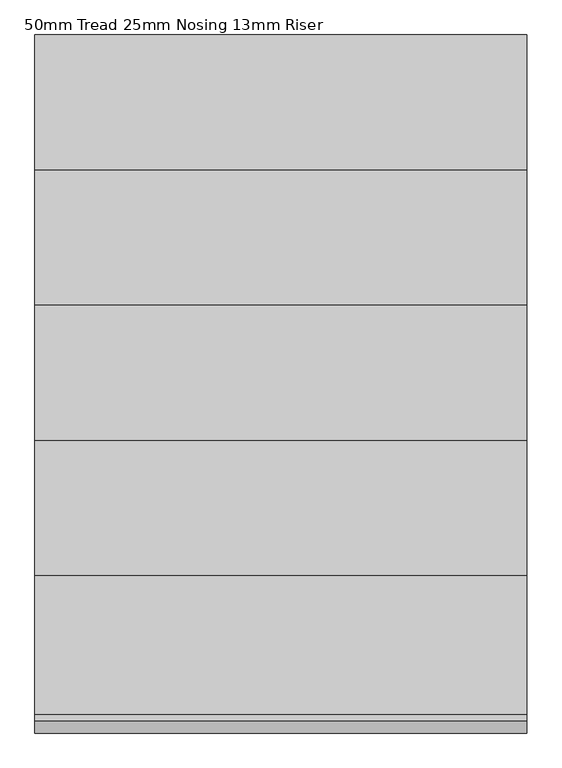
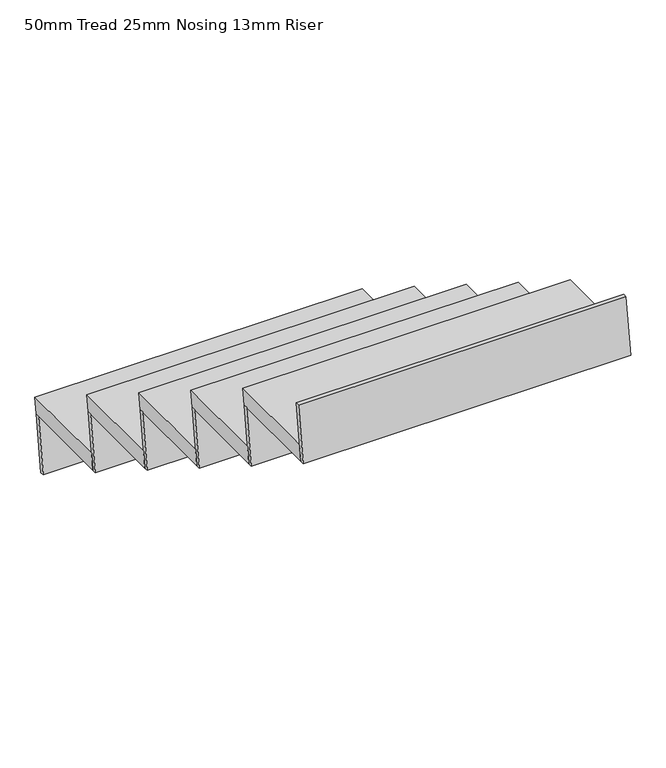
"""IFC4 building model written with IfcOpenShell, lengths in millimetres: stair flight geometry, 50mm Tread 25mm Nosing 13mm Riser."""

from ifc_helpers import new_model, si_unit, frame, origin, place, context, project, spatial, polyline, outline, extrude, source, transform, mapped, element, save


def stair_flight_50mm_tread_25mm_nosing_13mm_riser_46b24cc8(model_context):
    return source(origin(), model_context, "Body", "SweptSolid", [
        extrude(outline(polyline([(2452.4280728, 1739.1304348), (2752.4280728, 1739.1304348), (2745.2405728, 1689.1304348), (2445.2405728, 1689.1304348), (2452.4280728, 1739.1304348)])), frame((-10585.5805681, 0.0, 0.0), z_axis=(1.0, 0.0, 0.0), x_axis=(0.0, 1.0, 0.0)), (0.0, 0.0, 1.0), 1000.0257813),
        extrude(outline(polyline([(2745.2405728, 1689.1304348), (2720.2405728, 1515.2173913), (2707.6120828, 1515.2173913), (2732.6120828, 1689.1304348), (2745.2405728, 1689.1304348)])), frame((-10585.5805681, 0.0, 0.0), z_axis=(1.0, 0.0, 0.0), x_axis=(0.0, 1.0, 0.0)), (0.0, 0.0, 1.0), 1000.0257813),
        extrude(outline(polyline([(2470.2405728, 1863.0434783), (2445.2405728, 1689.1304348), (2432.6120828, 1689.1304348), (2457.6120828, 1863.0434783), (2470.2405728, 1863.0434783)])), frame((-10585.5805681, 0.0, 0.0), z_axis=(1.0, 0.0, 0.0), x_axis=(0.0, 1.0, 0.0)), (0.0, 0.0, 1.0), 1000.0257813),
        extrude(outline(polyline([(2177.4280728, 1913.0434783), (2477.4280728, 1913.0434783), (2470.2405728, 1863.0434783), (2170.2405728, 1863.0434783), (2177.4280728, 1913.0434783)])), frame((-10585.5805681, 0.0, 0.0), z_axis=(1.0, 0.0, 0.0), x_axis=(0.0, 1.0, 0.0)), (0.0, 0.0, 1.0), 1000.0257813),
        extrude(outline(polyline([(2195.2405728, 2036.9565217), (2170.2405728, 1863.0434783), (2157.6120828, 1863.0434783), (2182.6120828, 2036.9565217), (2195.2405728, 2036.9565217)])), frame((-10585.5805681, 0.0, 0.0), z_axis=(1.0, 0.0, 0.0), x_axis=(0.0, 1.0, 0.0)), (0.0, 0.0, 1.0), 1000.0257813),
        extrude(outline(polyline([(1902.4280728, 2086.9565217), (2202.4280728, 2086.9565217), (2195.2405728, 2036.9565217), (1895.2405728, 2036.9565217), (1902.4280728, 2086.9565217)])), frame((-10585.5805681, 0.0, 0.0), z_axis=(1.0, 0.0, 0.0), x_axis=(0.0, 1.0, 0.0)), (0.0, 0.0, 1.0), 1000.0257813),
        extrude(outline(polyline([(1920.2405728, 2210.8695652), (1895.2405728, 2036.9565217), (1882.6120828, 2036.9565217), (1907.6120828, 2210.8695652), (1920.2405728, 2210.8695652)])), frame((-10585.5805681, 0.0, 0.0), z_axis=(1.0, 0.0, 0.0), x_axis=(0.0, 1.0, 0.0)), (0.0, 0.0, 1.0), 1000.0257813),
        extrude(outline(polyline([(1627.4280728, 2260.8695652), (1927.4280728, 2260.8695652), (1920.2405728, 2210.8695652), (1620.2405728, 2210.8695652), (1627.4280728, 2260.8695652)])), frame((-10585.5805681, 0.0, 0.0), z_axis=(1.0, 0.0, 0.0), x_axis=(0.0, 1.0, 0.0)), (0.0, 0.0, 1.0), 1000.0257813),
        extrude(outline(polyline([(1645.2405728, 2384.7826087), (1620.2405728, 2210.8695652), (1607.6120828, 2210.8695652), (1632.6120828, 2384.7826087), (1645.2405728, 2384.7826087)])), frame((-10585.5805681, 0.0, 0.0), z_axis=(1.0, 0.0, 0.0), x_axis=(0.0, 1.0, 0.0)), (0.0, 0.0, 1.0), 1000.0257813),
        extrude(outline(polyline([(1370.2405728, 2558.6956522), (1345.2405728, 2384.7826087), (1332.6120828, 2384.7826087), (1357.6120828, 2558.6956522), (1370.2405728, 2558.6956522)])), frame((-10585.5805681, 0.0, 0.0), z_axis=(1.0, 0.0, 0.0), x_axis=(0.0, 1.0, 0.0)), (0.0, 0.0, 1.0), 1000.0257813),
        extrude(outline(polyline([(1352.4280728, 2434.7826087), (1652.4280728, 2434.7826087), (1645.2405728, 2384.7826087), (1345.2405728, 2384.7826087), (1352.4280728, 2434.7826087)])), frame((-10585.5805681, 0.0, 0.0), z_axis=(1.0, 0.0, 0.0), x_axis=(0.0, 1.0, 0.0)), (0.0, 0.0, 1.0), 1000.0257813),
    ])


if __name__ == "__main__":
    model = new_model("IFC4")
    model_context = context("Model", 3, world=origin())
    ifc_project = project(units=[si_unit("LENGTHUNIT", "METRE", prefix="MILLI")], contexts=[model_context])
    site = spatial("IfcSite", under=ifc_project)
    building = spatial("IfcBuilding", under=site)
    placement = place(None, origin())
    stair_flight_50mm_tread_25mm_nosing_13mm_riser_shape = stair_flight_50mm_tread_25mm_nosing_13mm_riser_46b24cc8(model_context)
    element("IfcStairFlight", 1, ObjectType="50mm Tread 25mm Nosing 13mm Riser", at=placement, inside=building, context=model_context, shape_type="MappedRepresentation", body=[
        mapped(stair_flight_50mm_tread_25mm_nosing_13mm_riser_shape, transform((0.0, 0.0, 0.0), x_axis=(1.0, 0.0, 0.0), y_axis=(0.0, 1.0, 0.0), z_axis=(0.0, 0.0, 1.0))),
    ])
    save(model, "model.ifc")
